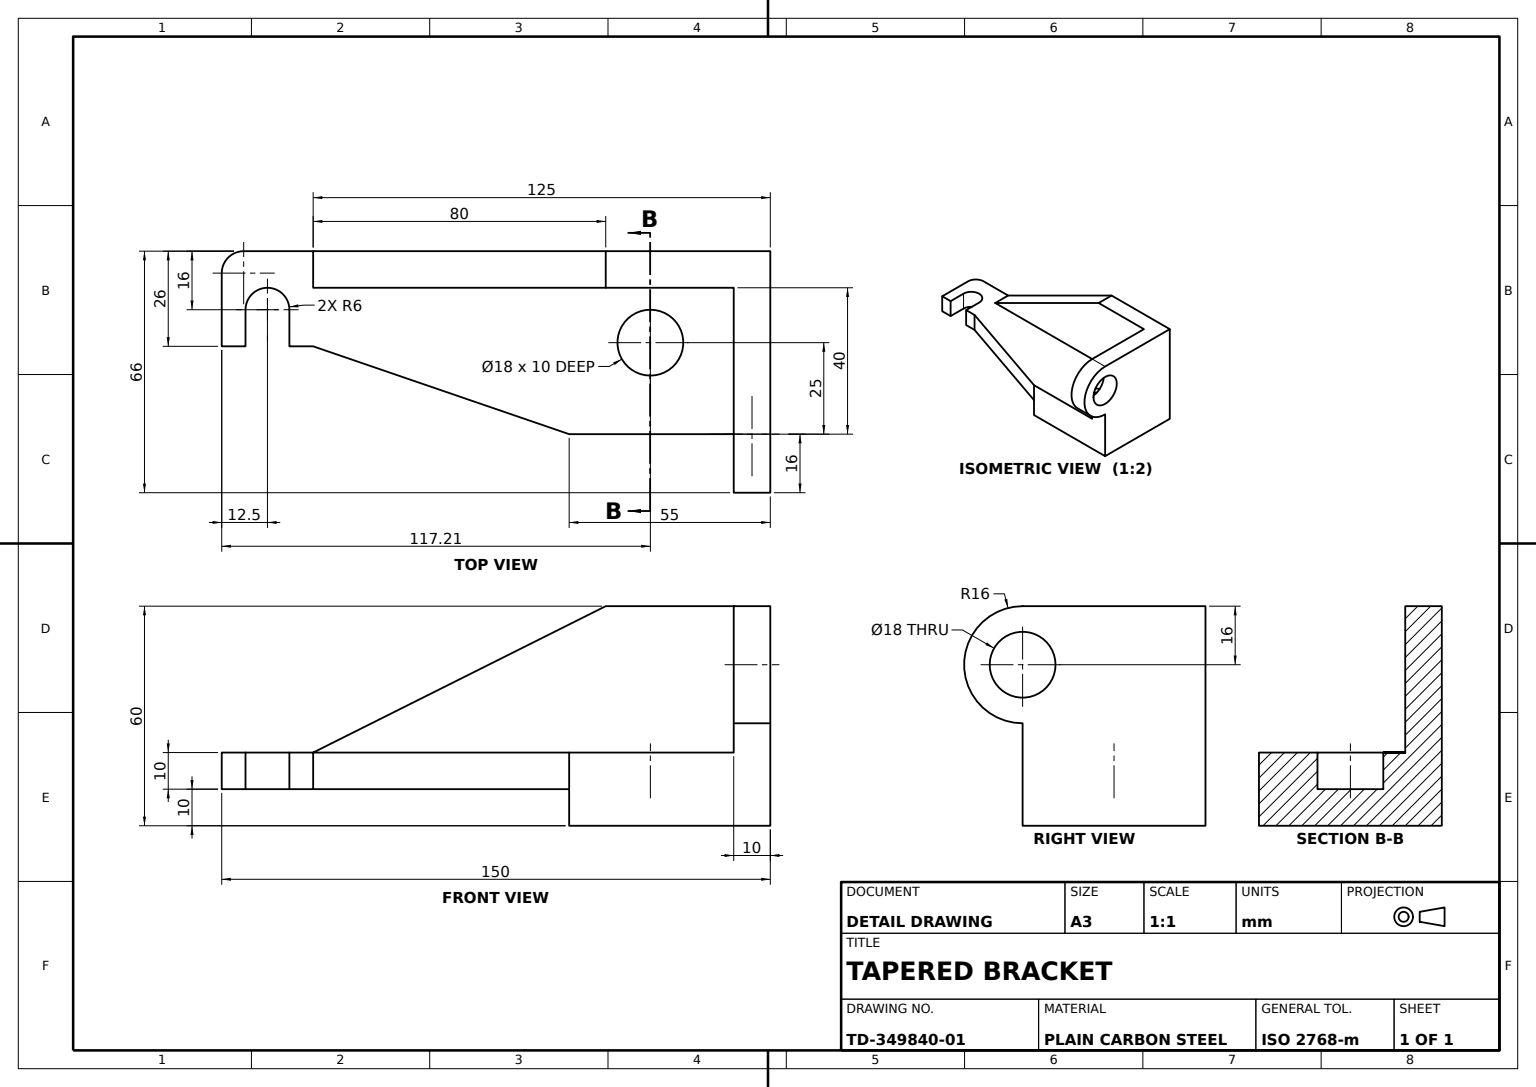
from build123d import *

# Parameters (mm, degrees)
BASE_PROFILE_DEPTH      = 10
SIDE_BLOCK_SKETCH_W     = 50
SIDE_BLOCK_SKETCH_H     = 50
SIDE_BLOCK_DEPTH        = 10
WEB_DEPTH               = 10
GUSSET_DEPTH            = 10
RAIL_SKETCH_W           = 55
RAIL_SKETCH_H           = 60
RAIL_DEPTH              = 10
POCKET_CUT_DEPTH        = 10
RELIEF_CUT_DEPTH        = 10
ARM_MOUNT_DEPTH         = 10
HOOK_ARM_DEPTH          = 10
RING_BOSS_DEPTH         = 10
BORE_18_SKETCH_R        = 9
BORE_18_DEPTH           = 10
HOOK_CUTOUT_18_SKETCH_R = 9
HOOK_CUTOUT_18_DEPTH    = 10


with BuildPart() as part:
    # Base Profile Sketch → Base Profile (new body)
    with BuildSketch(Plane.XY):
        Polygon((0, 0), (125, 0), (125, 40), (125, 50), (80, 50), (80, 10), (0, 10), align=None)
    extrude(amount=BASE_PROFILE_DEPTH)

    # Side Block Sketch → Side Block (add)
    with BuildSketch(Plane(origin=(125, 0, 0), x_dir=(0, 0, -1), z_dir=(1, 0, 0))):
        with Locations((-35, 25)):
            Rectangle(SIDE_BLOCK_SKETCH_W, SIDE_BLOCK_SKETCH_H)
    extrude(amount=-SIDE_BLOCK_DEPTH)

    # Web Sketch → Web (add)
    with BuildSketch(Plane.XZ):
        Polygon((115, 60), (70, 60), (0, 40), (0, 10), (115, 10), align=None)
    extrude(amount=-WEB_DEPTH)

    # Gusset Sketch → Gusset (add)
    with BuildSketch(Plane(origin=(0, 0, 0), x_dir=(-1, 0, 0), z_dir=(0, 0, -1))):
        Polygon((-80, 50), (0, 10), (-80, 10), align=None)
    extrude(amount=-GUSSET_DEPTH)

    # Rail Sketch → Rail (add)
    with BuildSketch(Plane.XZ):
        with Locations((97.5, 30)):
            Rectangle(RAIL_SKETCH_W, RAIL_SKETCH_H)
    extrude(amount=RAIL_DEPTH)

    # Pocket Cut Sketch → Pocket Cut (cut)
    with BuildSketch(Plane.XY.offset(60)):
        Polygon((115, 50), (125, 50), (125, -10), (70, -10), (70, 10), (115, 10), align=None)
    extrude(amount=-POCKET_CUT_DEPTH, mode=Mode.SUBTRACT)

    # Relief Cut Sketch → Relief Cut (cut)
    with BuildSketch(Plane(origin=(0, 10, 0), x_dir=(1, 0, 0), z_dir=(0, 1, 0))):
        Polygon((0, -40), (0, -10), (70, -10), (70, -60), align=None)
    extrude(amount=-RELIEF_CUT_DEPTH, mode=Mode.SUBTRACT)

    # Arm Mount Sketch → Arm Mount (add)
    with BuildSketch(Plane(origin=(0, 10, 0), x_dir=(1, 0, 0), z_dir=(0, 1, 0))):
        Polygon((70, -10), (0, -10), (0, -26), (70, -50), align=None)
    extrude(amount=-ARM_MOUNT_DEPTH)

    # Hook Arm Sketch → Hook Arm (add)
    with BuildSketch(Plane.XZ):
        with BuildLine():
            Line((0, 0), (-19, 0))
            ThreePointArc((-19, 0), (-23.242640687, 1.757359313), (-25, 6))
            Line((-25, 6), (-25, 26))
            Line((-25, 26), (-19, 26))
            Line((-19, 26), (-18.5, 26))
            Line((-18.5, 26), (-18.5, 16))
            ThreePointArc((-18.5, 16), (-12.5, 10), (-6.5, 16))
            Line((-6.5, 16), (-6.5, 26))
            Line((-6.5, 26), (-6, 26))
            Line((-6, 26), (0, 26))
            Line((0, 26), (0, 0))
        make_face()
    extrude(amount=-HOOK_ARM_DEPTH)

    # Ring Boss Sketch → Ring Boss (add)
    with BuildSketch(Plane(origin=(125, 0, 0), x_dir=(0, 0, -1), z_dir=(1, 0, 0))):
        with BuildLine():
            Line((-50, 50), (-50, 18))
            ThreePointArc((-50, 18), (-66, 34), (-50, 50))
        make_face()
    extrude(amount=-RING_BOSS_DEPTH)

    # Bore Ø18 Sketch → Bore Ø18 (cut)
    with BuildSketch(Plane(origin=(125, 0, 0), x_dir=(0, 0, -1), z_dir=(1, 0, 0))):
        with Locations((-50, 34)):
            Circle(BORE_18_SKETCH_R)
    extrude(amount=-BORE_18_DEPTH, mode=Mode.SUBTRACT)

    # Hook Cutout Ø18 Sketch → Hook Cutout Ø18 (cut)
    with BuildSketch(Plane(origin=(0, 10, 0), x_dir=(1, 0, 0), z_dir=(0, 1, 0))):
        with Locations(Location((92.205854711, -25, 0), (0, 0, 270))):
            Circle(HOOK_CUTOUT_18_SKETCH_R)
    extrude(amount=-HOOK_CUTOUT_18_DEPTH, mode=Mode.SUBTRACT)


solid = part.part
